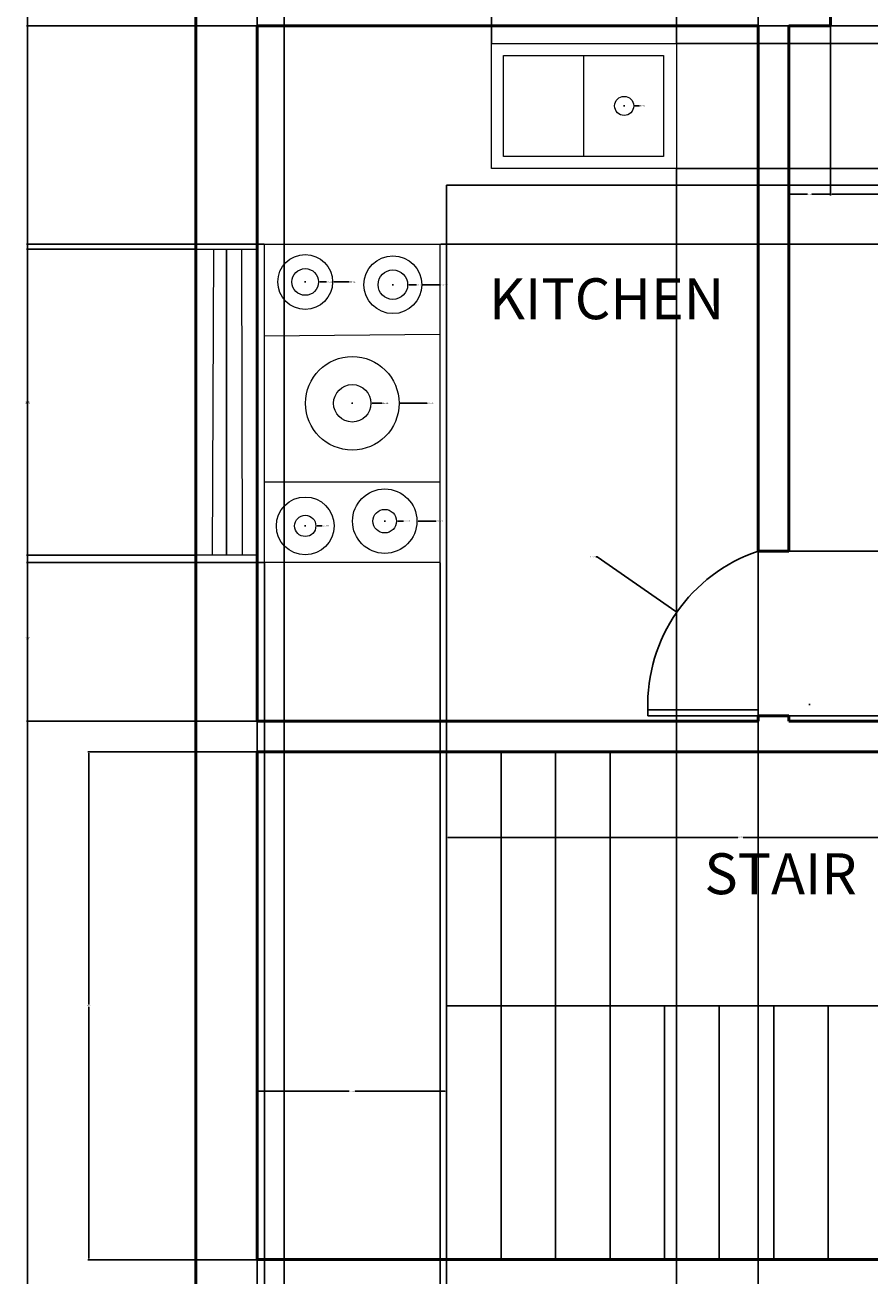
# Model space of a CAD drawing. Units: inches. Extents: x 1926 to 2293, y 1738 to 2280.
# Tile 3 of 6: x 1926 to 2050, y 1931 to 2114. Entities that reach past the tile are written whole.
import ezdxf

# ---------------------------------------------------------------- set-up
doc = ezdxf.new("R2010")
doc.units = ezdxf.units.IN
for name, color, linetype, lineweight in [('A-ANNO-DIMS', 2, 'Continuous', 18), ('A-AREA-IDEN', 7, 'Continuous', 25), ('A-DOOR', 3, 'Continuous', 25), ('A-EQPM', 8, 'Continuous', 18), ('A-FLOR-CASE', 9, 'Continuous', 25), ('A-FLOR-FIXT', 9, 'Continuous', 18), ('A-FLOR-STRS', 7, 'Continuous', 25), ('A-GLAZ', 4, 'Continuous', 18), ('A-WALL', 7, 'Continuous', 50)]:
    doc.layers.add(name, color=color, linetype=linetype, lineweight=lineweight)
doc.styles.get("Standard").update_dxf_attribs({"font": 'arial.ttf'})
doc.dimstyles.get("Standard").update_dxf_attribs({"dimtxt": 0.18, "dimasz": 0.18, "dimexe": 0.18, "dimexo": 0.0625, "dimgap": 0.09, "dimtad": 0, "dimtih": 1, "dimtoh": 1, "dimdec": 4, "dimzin": 0, "dimdsep": 46, "dimtxsty": 'Standard', "dimcen": 0.09, "dimadec": 0, "dimazin": 0, "dimtfac": 1, "dimtdec": 4, "dimtofl": 0, "dimtmove": 0, "dimatfit": 3, "dimfxl": 1, "dimtolj": 1, "dimtzin": 0, "dimarcsym": 0})

# ---------------------------------------------------------------- blocks, each defined once
blk = doc.blocks.new('*D39')
at = {"layer": 'A-ANNO-DIMS', "color": 0, "lineweight": -2, "transparency": 16777216}
for p, q in [((1959.69, 2007.66), (1934.88, 2007.66)), ((1935.06, 2007.48), (1935.06, 1970.59)), ((1935.06, 1933.34), (1935.06, 1970.23)), ((1959.69, 1933.16), (1934.88, 1933.16))]:
    blk.add_line(p, q, dxfattribs=at)
at = {"layer": 'A-ANNO-DIMS', "color": 0, "transparency": 16777216}
for points in [[(1935.03, 2007.48), (1935.09, 2007.48), (1935.06, 2007.66)], [(1935.03, 1933.34), (1935.09, 1933.34), (1935.06, 1933.16)]]:
    blk.add_solid(points, dxfattribs=at)
at = {"layer": 'Defpoints', "color": 0, "transparency": 16777216}
for p in [(1935.06, 2007.66), (1959.76, 2007.66), (1959.76, 1933.16)]:
    blk.add_point(p, dxfattribs=at)
at = {"layer": 'A-ANNO-DIMS', "color": 0, "transparency": 16777216, "insert": (1935.06, 1970.41), "char_height": 0.18, "attachment_point": 5}
blk.add_mtext('\\A1;74.5', dxfattribs=at)
blk = doc.blocks.new('*D40')
at = {"layer": 'A-ANNO-DIMS', "color": 0, "lineweight": -2, "transparency": 16777216}
for p, q in [((1959.69, 2114.16), (1925.88, 2114.16)), ((1926.06, 2113.98), (1926.06, 2063.34)), ((1926.06, 2012.34), (1926.06, 2062.98)), ((1959.69, 2012.16), (1925.88, 2012.16))]:
    blk.add_line(p, q, dxfattribs=at)
at = {"layer": 'A-ANNO-DIMS', "color": 0, "transparency": 16777216}
for points in [[(1926.03, 2113.98), (1926.09, 2113.98), (1926.06, 2114.16)], [(1926.03, 2012.34), (1926.09, 2012.34), (1926.06, 2012.16)]]:
    blk.add_solid(points, dxfattribs=at)
at = {"layer": 'Defpoints', "color": 0, "transparency": 16777216}
for p in [(1926.06, 2114.16), (1959.76, 2114.16), (1959.76, 2012.16)]:
    blk.add_point(p, dxfattribs=at)
at = {"layer": 'A-ANNO-DIMS', "color": 0, "transparency": 16777216, "insert": (1926.06, 2063.16), "char_height": 0.18, "attachment_point": 5}
blk.add_mtext('\\A1;102', dxfattribs=at)
blk = doc.blocks.new('*D46')
at = {"layer": 'A-ANNO-DIMS', "color": 0, "lineweight": -2, "transparency": 16777216}
for p, q in [((1959.76, 2114.22), (1959.76, 2280.04)), ((1959.94, 2279.86), (1996.18, 2279.86)), ((2033.08, 2279.86), (1996.83, 2279.86)), ((2033.26, 2114.22), (2033.26, 2280.04))]:
    blk.add_line(p, q, dxfattribs=at)
at = {"layer": 'A-ANNO-DIMS', "color": 0, "transparency": 16777216}
for points in [[(1959.94, 2279.89), (1959.94, 2279.83), (1959.76, 2279.86)], [(2033.08, 2279.89), (2033.08, 2279.83), (2033.26, 2279.86)]]:
    blk.add_solid(points, dxfattribs=at)
at = {"layer": 'Defpoints', "color": 0, "transparency": 16777216}
for p in [(2033.26, 2279.86), (1959.76, 2114.16), (2033.26, 2114.16)]:
    blk.add_point(p, dxfattribs=at)
at = {"layer": 'A-ANNO-DIMS', "color": 0, "transparency": 16777216, "insert": (1996.51, 2279.86), "char_height": 0.18, "attachment_point": 5}
blk.add_mtext('\\A1;73.5', dxfattribs=at)
blk = doc.blocks.new('*D47')
at = {"layer": 'A-ANNO-DIMS', "color": 0, "lineweight": -2, "transparency": 16777216}
for p, q in [((1950.76, 2036.47), (1950.76, 1737.97)), ((1959.76, 2036.47), (1959.76, 1737.97)), ((1950.94, 1738.15), (1955.11, 1738.15)), ((1959.58, 1738.15), (1955.41, 1738.15))]:
    blk.add_line(p, q, dxfattribs=at)
at = {"layer": 'A-ANNO-DIMS', "color": 0, "transparency": 16777216}
for points in [[(1950.94, 1738.18), (1950.94, 1738.12), (1950.76, 1738.15)], [(1959.58, 1738.18), (1959.58, 1738.12), (1959.76, 1738.15)]]:
    blk.add_solid(points, dxfattribs=at)
at = {"layer": 'Defpoints', "color": 0, "transparency": 16777216}
for p in [(1950.76, 2036.53), (1959.76, 2036.53), (1959.76, 1738.15)]:
    blk.add_point(p, dxfattribs=at)
at = {"layer": 'A-ANNO-DIMS', "color": 0, "transparency": 16777216, "insert": (1955.26, 1738.15), "char_height": 0.18, "attachment_point": 5}
blk.add_mtext('\\A1;9', dxfattribs=at)
blk = doc.blocks.new('*D48')
at = {"layer": 'A-ANNO-DIMS', "color": 0, "lineweight": -2, "transparency": 16777216}
for p, q in [((1950.69, 2036.53), (1925.88, 2036.53)), ((1926.06, 2036.35), (1926.06, 2024.53)), ((1926.06, 2012.34), (1926.06, 2024.16)), ((1959.69, 2012.16), (1925.88, 2012.16))]:
    blk.add_line(p, q, dxfattribs=at)
at = {"layer": 'A-ANNO-DIMS', "color": 0, "transparency": 16777216}
for points in [[(1926.03, 2036.35), (1926.09, 2036.35), (1926.06, 2036.53)], [(1926.03, 2012.34), (1926.09, 2012.34), (1926.06, 2012.16)]]:
    blk.add_solid(points, dxfattribs=at)
at = {"layer": 'Defpoints', "color": 0, "transparency": 16777216}
for p in [(1926.06, 2036.53), (1950.76, 2036.53), (1959.76, 2012.16)]:
    blk.add_point(p, dxfattribs=at)
at = {"layer": 'A-ANNO-DIMS', "color": 0, "transparency": 16777216, "insert": (1926.06, 2024.35), "char_height": 0.18, "attachment_point": 5}
blk.add_mtext('\\A1;24.367', dxfattribs=at)
blk = doc.blocks.new('*D49')
at = {"layer": 'A-ANNO-DIMS', "color": 0, "lineweight": -2, "transparency": 16777216}
for p, q in [((1950.69, 2081.42), (1925.88, 2081.42)), ((1926.06, 2081.24), (1926.06, 2059.16)), ((1926.06, 2036.71), (1926.06, 2058.79)), ((1950.69, 2036.53), (1925.88, 2036.53))]:
    blk.add_line(p, q, dxfattribs=at)
at = {"layer": 'A-ANNO-DIMS', "color": 0, "transparency": 16777216}
for points in [[(1926.03, 2081.24), (1926.09, 2081.24), (1926.06, 2081.42)], [(1926.03, 2036.71), (1926.09, 2036.71), (1926.06, 2036.53)]]:
    blk.add_solid(points, dxfattribs=at)
at = {"layer": 'Defpoints', "color": 0, "transparency": 16777216}
for p in [(1926.06, 2081.42), (1950.76, 2081.42), (1950.76, 2036.53)]:
    blk.add_point(p, dxfattribs=at)
at = {"layer": 'A-ANNO-DIMS', "color": 0, "transparency": 16777216, "insert": (1926.06, 2058.98), "char_height": 0.18, "attachment_point": 5}
blk.add_mtext('\\A1;44.89', dxfattribs=at)
blk = doc.blocks.new('*D50')
at = {"layer": 'A-ANNO-DIMS', "color": 0, "lineweight": -2, "transparency": 16777216}
for p, q in [((2033.32, 2037.09), (2281.64, 2037.09)), ((2281.46, 2036.91), (2281.46, 2025.19)), ((2281.46, 2013.1), (2281.46, 2024.83)), ((2033.32, 2012.92), (2281.64, 2012.92))]:
    blk.add_line(p, q, dxfattribs=at)
at = {"layer": 'A-ANNO-DIMS', "color": 0, "transparency": 16777216}
for points in [[(2281.43, 2036.91), (2281.49, 2036.91), (2281.46, 2037.09)], [(2281.43, 2013.1), (2281.49, 2013.1), (2281.46, 2012.92)]]:
    blk.add_solid(points, dxfattribs=at)
at = {"layer": 'Defpoints', "color": 0, "transparency": 16777216}
for p in [(2033.26, 2037.09), (2281.46, 2037.09), (2033.26, 2012.92)]:
    blk.add_point(p, dxfattribs=at)
at = {"layer": 'A-ANNO-DIMS', "color": 0, "transparency": 16777216, "insert": (2281.46, 2025.01), "char_height": 0.18, "attachment_point": 5}
blk.add_mtext('\\A1;24.17', dxfattribs=at)
blk = doc.blocks.new('*D51')
at = {"layer": 'A-ANNO-DIMS', "color": 0, "lineweight": -2, "transparency": 16777216}
for p, q in [((1959.76, 2012.1), (1959.76, 1737.97)), ((1987.52, 2012.1), (1987.52, 1737.97)), ((1959.94, 1738.15), (1973.24, 1738.15)), ((1987.34, 1738.15), (1974.03, 1738.15))]:
    blk.add_line(p, q, dxfattribs=at)
at = {"layer": 'A-ANNO-DIMS', "color": 0, "transparency": 16777216}
for points in [[(1959.94, 1738.18), (1959.94, 1738.12), (1959.76, 1738.15)], [(1987.34, 1738.18), (1987.34, 1738.12), (1987.52, 1738.15)]]:
    blk.add_solid(points, dxfattribs=at)
at = {"layer": 'Defpoints', "color": 0, "transparency": 16777216}
for p in [(1959.76, 2012.16), (1987.52, 2012.16), (1987.52, 1738.15)]:
    blk.add_point(p, dxfattribs=at)
at = {"layer": 'A-ANNO-DIMS', "color": 0, "transparency": 16777216, "insert": (1973.64, 1738.15), "char_height": 0.18, "attachment_point": 5}
blk.add_mtext('\\A1;27.76', dxfattribs=at)
blk = doc.blocks.new('*D52')
at = {"layer": 'A-ANNO-DIMS', "color": 0, "lineweight": -2, "transparency": 16777216}
for p, q in [((2033.32, 2114.16), (2281.64, 2114.16)), ((2281.46, 2113.98), (2281.46, 2102.67)), ((2281.46, 2090.99), (2281.46, 2102.31)), ((2033.32, 2090.81), (2281.64, 2090.81))]:
    blk.add_line(p, q, dxfattribs=at)
at = {"layer": 'A-ANNO-DIMS', "color": 0, "transparency": 16777216}
for points in [[(2281.43, 2113.98), (2281.49, 2113.98), (2281.46, 2114.16)], [(2281.43, 2090.99), (2281.49, 2090.99), (2281.46, 2090.81)]]:
    blk.add_solid(points, dxfattribs=at)
at = {"layer": 'Defpoints', "color": 0, "transparency": 16777216}
for p in [(2033.26, 2114.16), (2281.46, 2114.16), (2033.26, 2090.81)]:
    blk.add_point(p, dxfattribs=at)
at = {"layer": 'A-ANNO-DIMS', "color": 0, "transparency": 16777216, "insert": (2281.46, 2102.49), "char_height": 0.18, "attachment_point": 5}
blk.add_mtext('\\A1;23.348', dxfattribs=at)
blk = doc.blocks.new('*D53')
at = {"layer": 'A-ANNO-DIMS', "color": 0, "lineweight": -2, "transparency": 16777216}
for p, q in [((1994.13, 2111.62), (1994.13, 2280.04)), ((1994.31, 2279.86), (2007.3, 2279.86)), ((2021.07, 2279.86), (2008.09, 2279.86)), ((2021.25, 2111.62), (2021.25, 2280.04))]:
    blk.add_line(p, q, dxfattribs=at)
at = {"layer": 'A-ANNO-DIMS', "color": 0, "transparency": 16777216}
for points in [[(1994.31, 2279.89), (1994.31, 2279.83), (1994.13, 2279.86)], [(2021.07, 2279.89), (2021.07, 2279.83), (2021.25, 2279.86)]]:
    blk.add_solid(points, dxfattribs=at)
at = {"layer": 'Defpoints', "color": 0, "transparency": 16777216}
for p in [(2021.25, 2279.86), (1994.13, 2111.56), (2021.25, 2111.56)]:
    blk.add_point(p, dxfattribs=at)
at = {"layer": 'A-ANNO-DIMS', "color": 0, "transparency": 16777216, "insert": (2007.69, 2279.86), "char_height": 0.18, "attachment_point": 5}
blk.add_mtext('\\A1;27.13', dxfattribs=at)
blk = doc.blocks.new('*D54')
at = {"layer": 'A-ANNO-DIMS', "color": 0, "lineweight": -2, "transparency": 16777216}
for p, q in [((2021.32, 2111.56), (2281.64, 2111.56)), ((2281.46, 2111.38), (2281.46, 2102.58)), ((2281.46, 2093.41), (2281.46, 2102.21)), ((2021.32, 2093.23), (2281.64, 2093.23))]:
    blk.add_line(p, q, dxfattribs=at)
at = {"layer": 'A-ANNO-DIMS', "color": 0, "transparency": 16777216}
for points in [[(2281.43, 2111.38), (2281.49, 2111.38), (2281.46, 2111.56)], [(2281.43, 2093.41), (2281.49, 2093.41), (2281.46, 2093.23)]]:
    blk.add_solid(points, dxfattribs=at)
at = {"layer": 'Defpoints', "color": 0, "transparency": 16777216}
for p in [(2021.25, 2111.56), (2281.46, 2111.56), (2021.25, 2093.23)]:
    blk.add_point(p, dxfattribs=at)
at = {"layer": 'A-ANNO-DIMS', "color": 0, "transparency": 16777216, "insert": (2281.46, 2102.39), "char_height": 0.18, "attachment_point": 5}
blk.add_mtext('\\A1;18.332', dxfattribs=at)
blk = doc.blocks.new('*D55')
at = {"layer": 'A-ANNO-DIMS', "color": 0, "lineweight": -2, "transparency": 16777216}
for p, q in [((1960.83, 2035.38), (1960.83, 1737.97)), ((1986.57, 2035.38), (1986.57, 1737.97)), ((1961.01, 1738.15), (1973.3, 1738.15)), ((1986.39, 1738.15), (1974.09, 1738.15))]:
    blk.add_line(p, q, dxfattribs=at)
at = {"layer": 'A-ANNO-DIMS', "color": 0, "transparency": 16777216}
for points in [[(1961.01, 1738.18), (1961.01, 1738.12), (1960.83, 1738.15)], [(1986.39, 1738.18), (1986.39, 1738.12), (1986.57, 1738.15)]]:
    blk.add_solid(points, dxfattribs=at)
at = {"layer": 'Defpoints', "color": 0, "transparency": 16777216}
for p in [(1960.83, 2035.45), (1986.57, 2035.45), (1986.57, 1738.15)]:
    blk.add_point(p, dxfattribs=at)
at = {"layer": 'A-ANNO-DIMS', "color": 0, "transparency": 16777216, "insert": (1973.7, 1738.15), "char_height": 0.18, "attachment_point": 5}
blk.add_mtext('\\A1;25.74', dxfattribs=at)
blk = doc.blocks.new('*D56')
at = {"layer": 'A-ANNO-DIMS', "color": 0, "lineweight": -2, "transparency": 16777216}
for p, q in [((1960.76, 2082.13), (1925.88, 2082.13)), ((1926.06, 2081.95), (1926.06, 2058.97)), ((1926.06, 2035.63), (1926.06, 2058.61)), ((1960.76, 2035.45), (1925.88, 2035.45))]:
    blk.add_line(p, q, dxfattribs=at)
at = {"layer": 'A-ANNO-DIMS', "color": 0, "transparency": 16777216}
for points in [[(1926.03, 2081.95), (1926.09, 2081.95), (1926.06, 2082.13)], [(1926.03, 2035.63), (1926.09, 2035.63), (1926.06, 2035.45)]]:
    blk.add_solid(points, dxfattribs=at)
at = {"layer": 'Defpoints', "color": 0, "transparency": 16777216}
for p in [(1926.06, 2082.13), (1960.83, 2082.13), (1960.83, 2035.45)]:
    blk.add_point(p, dxfattribs=at)
at = {"layer": 'A-ANNO-DIMS', "color": 0, "transparency": 16777216, "insert": (1926.06, 2058.79), "char_height": 0.18, "attachment_point": 5}
blk.add_mtext('\\A1;46.69', dxfattribs=at)
blk = doc.blocks.new('*D57')
at = {"layer": 'A-ANNO-DIMS', "color": 0, "lineweight": -2, "transparency": 16777216}
for p, q in [((2021.25, 2093.16), (2021.25, 1737.97)), ((2033.26, 2090.75), (2033.26, 1737.97)), ((2021.43, 1738.15), (2026.8, 1738.15)), ((2033.08, 1738.15), (2027.71, 1738.15))]:
    blk.add_line(p, q, dxfattribs=at)
at = {"layer": 'A-ANNO-DIMS', "color": 0, "transparency": 16777216}
for points in [[(2021.43, 1738.18), (2021.43, 1738.12), (2021.25, 1738.15)], [(2033.08, 1738.18), (2033.08, 1738.12), (2033.26, 1738.15)]]:
    blk.add_solid(points, dxfattribs=at)
at = {"layer": 'Defpoints', "color": 0, "transparency": 16777216}
for p in [(2021.25, 2093.23), (2033.26, 2090.81), (2033.26, 1738.15)]:
    blk.add_point(p, dxfattribs=at)
at = {"layer": 'A-ANNO-DIMS', "color": 0, "transparency": 16777216, "insert": (2027.26, 1738.15), "char_height": 0.18, "attachment_point": 5}
blk.add_mtext('\\A1;12.002', dxfattribs=at)
blk = doc.blocks.new('*D58')
at = {"layer": 'A-ANNO-DIMS', "color": 0, "lineweight": -2, "transparency": 16777216}
for p, q in [((1987.58, 2090.81), (2281.64, 2090.81)), ((2281.46, 2090.63), (2281.46, 2086.66)), ((2281.46, 2082.31), (2281.46, 2086.29)), ((1986.63, 2082.13), (2281.64, 2082.13))]:
    blk.add_line(p, q, dxfattribs=at)
at = {"layer": 'A-ANNO-DIMS', "color": 0, "transparency": 16777216}
for points in [[(2281.43, 2090.63), (2281.49, 2090.63), (2281.46, 2090.81)], [(2281.43, 2082.31), (2281.49, 2082.31), (2281.46, 2082.13)]]:
    blk.add_solid(points, dxfattribs=at)
at = {"layer": 'Defpoints', "color": 0, "transparency": 16777216}
for p in [(1987.52, 2090.81), (2281.46, 2090.81), (1986.57, 2082.13)]:
    blk.add_point(p, dxfattribs=at)
at = {"layer": 'A-ANNO-DIMS', "color": 0, "transparency": 16777216, "insert": (2281.46, 2086.47), "char_height": 0.18, "attachment_point": 5}
blk.add_mtext('\\A1;8.682', dxfattribs=at)
blk = doc.blocks.new('*D63')
at = {"layer": 'A-ANNO-DIMS', "color": 0, "lineweight": -2, "transparency": 16777216}
for p, q in [((2043.88, 2114.1), (2043.88, 2089.28)), ((2073.61, 2114.1), (2073.61, 2089.28)), ((2044.06, 2089.46), (2058.35, 2089.46)), ((2073.43, 2089.46), (2059.14, 2089.46))]:
    blk.add_line(p, q, dxfattribs=at)
at = {"layer": 'A-ANNO-DIMS', "color": 0, "transparency": 16777216}
for points in [[(2044.06, 2089.49), (2044.06, 2089.43), (2043.88, 2089.46)], [(2073.43, 2089.49), (2073.43, 2089.43), (2073.61, 2089.46)]]:
    blk.add_solid(points, dxfattribs=at)
at = {"layer": 'Defpoints', "color": 0, "transparency": 16777216}
for p in [(2043.88, 2114.16), (2073.61, 2114.16), (2043.88, 2089.46)]:
    blk.add_point(p, dxfattribs=at)
at = {"layer": 'A-ANNO-DIMS', "color": 0, "transparency": 16777216, "insert": (2058.74, 2089.46), "char_height": 0.18, "attachment_point": 5}
blk.add_mtext('\\A1;29.73', dxfattribs=at)
blk = doc.blocks.new('*D64')
at = {"layer": 'A-ANNO-DIMS', "color": 0, "lineweight": -2, "transparency": 16777216}
for p, q in [((2037.76, 2114.1), (2037.76, 2089.28)), ((2043.88, 2114.1), (2043.88, 2089.28)), ((2037.94, 2089.46), (2040.49, 2089.46)), ((2043.7, 2089.46), (2041.14, 2089.46))]:
    blk.add_line(p, q, dxfattribs=at)
at = {"layer": 'A-ANNO-DIMS', "color": 0, "transparency": 16777216}
for points in [[(2037.94, 2089.49), (2037.94, 2089.43), (2037.76, 2089.46)], [(2043.7, 2089.49), (2043.7, 2089.43), (2043.88, 2089.46)]]:
    blk.add_solid(points, dxfattribs=at)
at = {"layer": 'Defpoints', "color": 0, "transparency": 16777216}
for p in [(2037.76, 2114.16), (2043.88, 2114.16), (2037.76, 2089.46)]:
    blk.add_point(p, dxfattribs=at)
at = {"layer": 'A-ANNO-DIMS', "color": 0, "transparency": 16777216, "insert": (2040.82, 2089.46), "char_height": 0.18, "attachment_point": 5}
blk.add_mtext('\\A1;6.12', dxfattribs=at)
blk = doc.blocks.new('*D68')
at = {"layer": 'A-ANNO-DIMS', "color": 0, "lineweight": -2, "transparency": 16777216}
for p, q in [((1959.76, 1933.22), (1959.76, 1958.04)), ((1959.94, 1957.86), (1973.18, 1957.86)), ((1987.35, 1957.86), (1974.11, 1957.86)), ((1987.53, 1933.22), (1987.53, 1958.04))]:
    blk.add_line(p, q, dxfattribs=at)
at = {"layer": 'A-ANNO-DIMS', "color": 0, "transparency": 16777216}
for points in [[(1959.94, 1957.89), (1959.94, 1957.83), (1959.76, 1957.86)], [(1987.35, 1957.89), (1987.35, 1957.83), (1987.53, 1957.86)]]:
    blk.add_solid(points, dxfattribs=at)
at = {"layer": 'Defpoints', "color": 0, "transparency": 16777216}
for p in [(1987.53, 1957.86), (1959.76, 1933.16), (1987.53, 1933.16)]:
    blk.add_point(p, dxfattribs=at)
at = {"layer": 'A-ANNO-DIMS', "color": 0, "transparency": 16777216, "insert": (1973.64, 1957.86), "char_height": 0.18, "attachment_point": 5}
blk.add_mtext('\\A1;27.774', dxfattribs=at)
blk = doc.blocks.new('*D69')
at = {"layer": 'A-ANNO-DIMS', "color": 0, "lineweight": -2, "transparency": 16777216}
for p, q in [((1987.53, 1970.47), (1987.53, 1995.29)), ((2073.75, 1970.47), (2073.75, 1995.29)), ((1987.71, 1995.11), (2030.25, 1995.11)), ((2073.57, 1995.11), (2031.03, 1995.11))]:
    blk.add_line(p, q, dxfattribs=at)
at = {"layer": 'A-ANNO-DIMS', "color": 0, "transparency": 16777216}
for points in [[(1987.71, 1995.14), (1987.71, 1995.08), (1987.53, 1995.11)], [(2073.57, 1995.14), (2073.57, 1995.08), (2073.75, 1995.11)]]:
    blk.add_solid(points, dxfattribs=at)
at = {"layer": 'Defpoints', "color": 0, "transparency": 16777216}
for p in [(2073.75, 1995.11), (1987.53, 1970.41), (2073.75, 1970.41)]:
    blk.add_point(p, dxfattribs=at)
at = {"layer": 'A-ANNO-DIMS', "color": 0, "transparency": 16777216, "insert": (2030.64, 1995.11), "char_height": 0.18, "attachment_point": 5}
blk.add_mtext('\\A1;86.22', dxfattribs=at)
blk = doc.blocks.new('*D79')
at = {"layer": 'A-ANNO-DIMS', "color": 0, "lineweight": -2, "transparency": 16777216}
for p, q in [((1959.76, 1833.35), (1959.76, 2280.04)), ((1959.94, 2279.86), (1961.41, 2279.86)), ((1963.53, 2279.86), (1962.06, 2279.86)), ((1963.71, 1828.81), (1963.71, 2280.04))]:
    blk.add_line(p, q, dxfattribs=at)
at = {"layer": 'A-ANNO-DIMS', "color": 0, "transparency": 16777216}
for points in [[(1959.94, 2279.89), (1959.94, 2279.83), (1959.76, 2279.86)], [(1963.53, 2279.89), (1963.53, 2279.83), (1963.71, 2279.86)]]:
    blk.add_solid(points, dxfattribs=at)
at = {"layer": 'Defpoints', "color": 0, "transparency": 16777216}
for p in [(1959.76, 2279.86), (1959.76, 1833.29), (1963.71, 1828.75)]:
    blk.add_point(p, dxfattribs=at)
at = {"layer": 'A-ANNO-DIMS', "color": 0, "transparency": 16777216, "insert": (1961.74, 2279.86), "char_height": 0.18, "attachment_point": 5}
blk.add_mtext('\\A1;3.96', dxfattribs=at)
blk = doc.blocks.new('*D85')
at = {"layer": 'A-ANNO-DIMS', "color": 0, "lineweight": -2, "transparency": 16777216}
for p, q in [((1950.69, 2255.16), (1925.88, 2255.16)), ((1926.06, 2254.98), (1926.06, 2024.34)), ((1926.06, 1793.34), (1926.06, 2023.98)), ((1950.69, 1793.16), (1925.88, 1793.16))]:
    blk.add_line(p, q, dxfattribs=at)
at = {"layer": 'A-ANNO-DIMS', "color": 0, "transparency": 16777216}
for points in [[(1926.03, 2254.98), (1926.09, 2254.98), (1926.06, 2255.16)], [(1926.03, 1793.34), (1926.09, 1793.34), (1926.06, 1793.16)]]:
    blk.add_solid(points, dxfattribs=at)
at = {"layer": 'Defpoints', "color": 0, "transparency": 16777216}
for p in [(1926.06, 2255.16), (1950.76, 2255.16), (1950.76, 1793.16)]:
    blk.add_point(p, dxfattribs=at)
at = {"layer": 'A-ANNO-DIMS', "color": 0, "transparency": 16777216, "insert": (1926.06, 2024.16), "char_height": 0.18, "attachment_point": 5}
blk.add_mtext('\\A1;462', dxfattribs=at)
blk = doc.blocks.new('*D88')
at = {"layer": 'A-ANNO-DIMS', "color": 0, "lineweight": -2, "transparency": 16777216}
for p, q in [((2072.97, 1939.43), (2073.15, 1939.43)), ((2073.06, 1939.34), (2073.06, 1939.52)), ((2043.15, 1883.11), (2054.28, 1904.07)), ((2042.97, 1883.11), (2043.15, 1883.11))]:
    blk.add_line(p, q, dxfattribs=at)
at = {"layer": 'A-ANNO-DIMS', "color": 0, "transparency": 16777216}
blk.add_solid([(2054.26, 1904.08), (2054.31, 1904.06), (2054.37, 1904.23)], dxfattribs=at)
at = {"layer": 'Defpoints', "color": 0, "transparency": 16777216}
for p in [(2073.06, 1939.43), (2054.37, 1904.23)]:
    blk.add_point(p, dxfattribs=at)
at = {"layer": 'A-ANNO-DIMS', "color": 0, "transparency": 16777216, "insert": (2042.49, 1883.11), "char_height": 0.18, "attachment_point": 5}
blk.add_mtext('\\A1;R39.85', dxfattribs=at)
blk = doc.blocks.new('*D91')
at = {"layer": 'A-ANNO-DIMS', "color": 0, "lineweight": -2, "transparency": 16777216}
for p, q in [((2009.43, 2036.26), (2009.61, 2036.26)), ((2009.61, 2036.26), (2021.15, 2028.24)), ((2040.69, 2014.59), (2040.87, 2014.59)), ((2040.78, 2014.5), (2040.78, 2014.68))]:
    blk.add_line(p, q, dxfattribs=at)
at = {"layer": 'A-ANNO-DIMS', "color": 0, "transparency": 16777216}
blk.add_solid([(2021.17, 2028.26), (2021.13, 2028.21), (2021.3, 2028.13)], dxfattribs=at)
at = {"layer": 'Defpoints', "color": 0, "transparency": 16777216}
for p in [(2021.3, 2028.13), (2040.78, 2014.59)]:
    blk.add_point(p, dxfattribs=at)
at = {"layer": 'A-ANNO-DIMS', "color": 0, "transparency": 16777216, "insert": (2008.95, 2036.26), "char_height": 0.18, "attachment_point": 5}
blk.add_mtext('\\A1;R23.72', dxfattribs=at)
blk = doc.blocks.new('*D93')
at = {"layer": 'A-ANNO-DIMS', "color": 0, "lineweight": -2, "transparency": 16777216}
for p, q in [((1973.61, 2058.79), (1973.79, 2058.79)), ((1973.7, 2058.7), (1973.7, 2058.88)), ((1984.67, 2058.79), (1980.74, 2058.79))]:
    blk.add_line(p, q, dxfattribs=at)
at = {"layer": 'A-ANNO-DIMS', "color": 0, "transparency": 16777216}
blk.add_solid([(1980.74, 2058.82), (1980.74, 2058.76), (1980.56, 2058.79)], dxfattribs=at)
at = {"layer": 'Defpoints', "color": 0, "transparency": 16777216}
for p in [(1966.84, 2058.79), (1980.56, 2058.79)]:
    blk.add_point(p, dxfattribs=at)
at = {"layer": 'A-ANNO-DIMS', "color": 0, "transparency": 16777216, "insert": (1985.16, 2058.79), "char_height": 0.18, "attachment_point": 5}
blk.add_mtext('\\A1;∅13.72', dxfattribs=at)
blk = doc.blocks.new('*D94')
at = {"layer": 'A-ANNO-DIMS', "color": 0, "lineweight": -2, "transparency": 16777216}
for p, q in [((2013.5, 2102.42), (2013.68, 2102.42)), ((2013.59, 2102.33), (2013.59, 2102.51)), ((2015.83, 2102.45), (2015.17, 2102.44))]:
    blk.add_line(p, q, dxfattribs=at)
at = {"layer": 'A-ANNO-DIMS', "color": 0, "transparency": 16777216}
blk.add_solid([(2015.17, 2102.47), (2015.17, 2102.41), (2014.99, 2102.44)], dxfattribs=at)
at = {"layer": 'Defpoints', "color": 0, "transparency": 16777216}
for p in [(2012.19, 2102.4), (2014.99, 2102.44)]:
    blk.add_point(p, dxfattribs=at)
at = {"layer": 'A-ANNO-DIMS', "color": 0, "transparency": 16777216, "insert": (2016.26, 2102.45), "char_height": 0.18, "attachment_point": 5}
blk.add_mtext('\\A1;∅2.80', dxfattribs=at)
blk = doc.blocks.new('*D95')
at = {"layer": 'A-ANNO-DIMS', "color": 0, "lineweight": -2, "transparency": 16777216}
for p, q in [((1966.7, 2076.59), (1966.88, 2076.59)), ((1966.79, 2076.5), (1966.79, 2076.68)), ((1973.23, 2076.59), (1971, 2076.59))]:
    blk.add_line(p, q, dxfattribs=at)
at = {"layer": 'A-ANNO-DIMS', "color": 0, "transparency": 16777216}
blk.add_solid([(1971, 2076.62), (1971, 2076.56), (1970.82, 2076.59)], dxfattribs=at)
at = {"layer": 'Defpoints', "color": 0, "transparency": 16777216}
for p in [(1962.77, 2076.59), (1970.82, 2076.59)]:
    blk.add_point(p, dxfattribs=at)
at = {"layer": 'A-ANNO-DIMS', "color": 0, "transparency": 16777216, "insert": (1973.72, 2076.59), "char_height": 0.18, "attachment_point": 5}
blk.add_mtext('\\A1;∅8.044', dxfattribs=at)
blk = doc.blocks.new('*D96')
at = {"layer": 'A-ANNO-DIMS', "color": 0, "lineweight": -2, "transparency": 16777216}
for p, q in [((1966.7, 2076.59), (1966.88, 2076.59)), ((1966.79, 2076.5), (1966.79, 2076.68)), ((1969.93, 2076.59), (1968.93, 2076.59))]:
    blk.add_line(p, q, dxfattribs=at)
at = {"layer": 'A-ANNO-DIMS', "color": 0, "transparency": 16777216}
blk.add_solid([(1968.93, 2076.62), (1968.93, 2076.56), (1968.75, 2076.59)], dxfattribs=at)
at = {"layer": 'Defpoints', "color": 0, "transparency": 16777216}
for p in [(1964.84, 2076.59), (1968.75, 2076.59)]:
    blk.add_point(p, dxfattribs=at)
at = {"layer": 'A-ANNO-DIMS', "color": 0, "transparency": 16777216, "insert": (1970.42, 2076.59), "char_height": 0.18, "attachment_point": 5}
blk.add_mtext('\\A1;∅3.916', dxfattribs=at)
blk = doc.blocks.new('*D97')
at = {"layer": 'A-ANNO-DIMS', "color": 0, "lineweight": -2, "transparency": 16777216}
for p, q in [((1979.57, 2076.19), (1979.75, 2076.19)), ((1979.66, 2076.1), (1979.66, 2076.28)), ((1986.44, 2076.17), (1984.07, 2076.18))]:
    blk.add_line(p, q, dxfattribs=at)
at = {"layer": 'A-ANNO-DIMS', "color": 0, "transparency": 16777216}
blk.add_solid([(1984.07, 2076.21), (1984.07, 2076.15), (1983.89, 2076.18)], dxfattribs=at)
at = {"layer": 'Defpoints', "color": 0, "transparency": 16777216}
for p in [(1975.42, 2076.2), (1983.89, 2076.18)]:
    blk.add_point(p, dxfattribs=at)
at = {"layer": 'A-ANNO-DIMS', "color": 0, "transparency": 16777216, "insert": (1987.12, 2076.17), "char_height": 0.18, "attachment_point": 5}
blk.add_mtext('\\A1;2X ∅8.478', dxfattribs=at)
blk = doc.blocks.new('*D98')
at = {"layer": 'A-ANNO-DIMS', "color": 0, "lineweight": -2, "transparency": 16777216}
for p, q in [((1979.57, 2076.19), (1979.75, 2076.19)), ((1979.66, 2076.1), (1979.66, 2076.28)), ((1983.12, 2076.17), (1982, 2076.18))]:
    blk.add_line(p, q, dxfattribs=at)
at = {"layer": 'A-ANNO-DIMS', "color": 0, "transparency": 16777216}
blk.add_solid([(1982, 2076.21), (1982, 2076.15), (1981.82, 2076.18)], dxfattribs=at)
at = {"layer": 'Defpoints', "color": 0, "transparency": 16777216}
for p in [(1977.49, 2076.2), (1981.82, 2076.18)]:
    blk.add_point(p, dxfattribs=at)
at = {"layer": 'A-ANNO-DIMS', "color": 0, "transparency": 16777216, "insert": (1983.62, 2076.17), "char_height": 0.18, "attachment_point": 5}
blk.add_mtext('\\A1;∅4.335', dxfattribs=at)
blk = doc.blocks.new('*D99')
at = {"layer": 'A-ANNO-DIMS', "color": 0, "lineweight": -2, "transparency": 16777216}
for p, q in [((1973.61, 2058.79), (1973.79, 2058.79)), ((1973.7, 2058.7), (1973.7, 2058.88)), ((1978.09, 2058.79), (1976.62, 2058.79))]:
    blk.add_line(p, q, dxfattribs=at)
at = {"layer": 'A-ANNO-DIMS', "color": 0, "transparency": 16777216}
blk.add_solid([(1976.62, 2058.82), (1976.62, 2058.76), (1976.44, 2058.79)], dxfattribs=at)
at = {"layer": 'Defpoints', "color": 0, "transparency": 16777216}
for p in [(1970.95, 2058.79), (1976.44, 2058.79)]:
    blk.add_point(p, dxfattribs=at)
at = {"layer": 'A-ANNO-DIMS', "color": 0, "transparency": 16777216, "insert": (1978.56, 2058.79), "char_height": 0.18, "attachment_point": 5}
blk.add_mtext('\\A1;∅5.491', dxfattribs=at)
blk = doc.blocks.new('*D100')
at = {"layer": 'A-ANNO-DIMS', "color": 0, "lineweight": -2, "transparency": 16777216}
for p, q in [((1966.71, 2040.8), (1966.89, 2040.8)), ((1966.8, 2040.71), (1966.8, 2040.89)), ((1969.29, 2040.83), (1968.53, 2040.82))]:
    blk.add_line(p, q, dxfattribs=at)
at = {"layer": 'A-ANNO-DIMS', "color": 0, "transparency": 16777216}
blk.add_solid([(1968.53, 2040.85), (1968.53, 2040.79), (1968.35, 2040.82)], dxfattribs=at)
at = {"layer": 'Defpoints', "color": 0, "transparency": 16777216}
for p in [(1965.24, 2040.78), (1968.35, 2040.82)]:
    blk.add_point(p, dxfattribs=at)
at = {"layer": 'A-ANNO-DIMS', "color": 0, "transparency": 16777216, "insert": (1969.78, 2040.83), "char_height": 0.18, "attachment_point": 5}
blk.add_mtext('\\A1;∅3.114', dxfattribs=at)
blk = doc.blocks.new('*D101')
at = {"layer": 'A-ANNO-DIMS', "color": 0, "lineweight": -2, "transparency": 16777216}
for p, q in [((1978.37, 2041.5), (1978.55, 2041.5)), ((1978.46, 2041.41), (1978.46, 2041.59)), ((1986.02, 2041.52), (1983.36, 2041.51))]:
    blk.add_line(p, q, dxfattribs=at)
at = {"layer": 'A-ANNO-DIMS', "color": 0, "transparency": 16777216}
blk.add_solid([(1983.36, 2041.54), (1983.36, 2041.48), (1983.18, 2041.51)], dxfattribs=at)
at = {"layer": 'Defpoints', "color": 0, "transparency": 16777216}
for p in [(1973.74, 2041.49), (1983.18, 2041.51)]:
    blk.add_point(p, dxfattribs=at)
at = {"layer": 'A-ANNO-DIMS', "color": 0, "transparency": 16777216, "insert": (1986.51, 2041.52), "char_height": 0.18, "attachment_point": 5}
blk.add_mtext('\\A1;∅9.444', dxfattribs=at)
blk = doc.blocks.new('*D102')
at = {"layer": 'A-ANNO-DIMS', "color": 0, "lineweight": -2, "transparency": 16777216}
for p, q in [((1978.37, 2041.5), (1978.55, 2041.5)), ((1978.46, 2041.41), (1978.46, 2041.59)), ((1981.23, 2041.52), (1980.37, 2041.51))]:
    blk.add_line(p, q, dxfattribs=at)
at = {"layer": 'A-ANNO-DIMS', "color": 0, "transparency": 16777216}
blk.add_solid([(1980.37, 2041.54), (1980.37, 2041.48), (1980.19, 2041.51)], dxfattribs=at)
at = {"layer": 'Defpoints', "color": 0, "transparency": 16777216}
for p in [(1976.73, 2041.49), (1980.19, 2041.51)]:
    blk.add_point(p, dxfattribs=at)
at = {"layer": 'A-ANNO-DIMS', "color": 0, "transparency": 16777216, "insert": (1981.72, 2041.52), "char_height": 0.18, "attachment_point": 5}
blk.add_mtext('\\A1;∅3.459', dxfattribs=at)

msp = doc.modelspace()

# ---------------------------------------------------------------- linework, layer by layer
at = {"layer": 'A-DOOR'}
for p, q in [((2017.0689, 2012.9217), (2017.0689, 2013.8047)), ((2017.0689, 2013.8047), (2033.2569, 2013.8047)), ((2033.2569, 2013.8047), (2033.2569, 2012.9217)), ((2033.2569, 2012.9217), (2017.0689, 2012.9217))]:
    msp.add_line(p, q, dxfattribs=at)
msp.add_arc((2040.7776, 2014.5946), 23.7219, 108.483967, 181.908063, dxfattribs=at)
at = {"layer": 'A-EQPM'}
for p, q in [((1960.8266, 2068.7118), (1986.5655, 2068.911)), ((1960.8266, 2047.2934), (1986.5655, 2047.2934))]:
    msp.add_line(p, q, dxfattribs=at)
msp.add_lwpolyline([(1960.8266, 2082.133), (1986.5655, 2082.133), (1986.5655, 2035.4453), (1960.8266, 2035.4453)], close=True, dxfattribs=at)
for centre, radius in [((1966.7946, 2076.5885), 4.0222), ((1979.6559, 2076.19), 4.2388), ((1966.7946, 2076.5885), 1.9581), ((1979.6559, 2076.19), 2.1674), ((1973.696, 2058.7891), 6.8607), ((1973.696, 2058.7891), 2.7456), ((1966.7969, 2040.8011), 4.2388), ((1978.4618, 2041.4985), 4.722), ((1978.4618, 2041.4985), 1.7297), ((1966.7969, 2040.8011), 1.5571)]:
    msp.add_circle(centre, radius, dxfattribs=at)
at = {"layer": 'A-FLOR-CASE'}
for p, q in [((1987.5186, 2012.1622), (1987.5186, 2090.8146)), ((1987.5186, 2090.8146), (2033.2569, 2090.8146))]:
    msp.add_line(p, q, dxfattribs=at)
at = {"layer": 'A-FLOR-FIXT'}
msp.add_line((2007.624, 2109.8164), (2007.624, 2095.0195), dxfattribs=at)
for points in [[(1994.1266, 2111.5596), (2021.2546, 2111.5596), (2021.2546, 2093.2275), (1994.1266, 2093.2275)], [(1995.8924, 2109.8164), (2019.3556, 2109.8164), (2019.3556, 2095.0195), (1995.8924, 2095.0195)]]:
    msp.add_lwpolyline(points, close=True, dxfattribs=at)
msp.add_circle((2013.5904, 2102.418), 1.4023, dxfattribs=at)
at = {"layer": 'A-FLOR-STRS'}
for p, q in [((1987.531, 2007.6622), (1987.531, 1933.1622)), ((1995.531, 2007.6622), (1995.531, 1933.1622)), ((2003.531, 2007.6622), (2003.531, 1933.1622)), ((2011.531, 2007.6622), (2011.531, 1933.1622)), ((1987.531, 1970.4122), (2073.7521, 1970.4122)), ((2019.531, 1970.4122), (2019.531, 1933.1622)), ((2027.531, 1970.4122), (2027.531, 1933.1622)), ((2035.531, 1970.4122), (2035.531, 1933.1622)), ((2043.531, 1970.4122), (2043.531, 1933.1622))]:
    msp.add_line(p, q, dxfattribs=at)
at = {"layer": 'A-GLAZ'}
for p, q in [((1953.1897, 2036.5292), (1953.3811, 2081.4221)), ((1957.5911, 2036.5292), (1957.4954, 2081.4221))]:
    msp.add_line(p, q, dxfattribs=at)
for points in [[(1950.7569, 2081.4221), (1959.7569, 2081.4221), (1959.7569, 2036.5292), (1950.7569, 2036.5292)], [(1955.2569, 2081.4221), (1955.2569, 2081.4221), (1955.2569, 2036.5292), (1955.2569, 2036.5292)]]:
    msp.add_lwpolyline(points, close=True, dxfattribs=at)
at = {"layer": 'A-WALL'}
for p, q in [((1950.7569, 1793.1622), (1950.7569, 2255.1622)), ((2043.8774, 2114.1622), (2043.8774, 2118.6622)), ((1959.7569, 2114.1622), (2033.2569, 2114.1622)), ((1959.7569, 2012.1622), (1959.7569, 2114.1622)), ((2033.2569, 2037.0927), (2033.2569, 2114.1622)), ((2037.7569, 2114.1622), (2043.8774, 2114.1622)), ((2037.7569, 2037.0927), (2037.7569, 2114.1622)), ((2033.2569, 2037.0927), (2037.7569, 2037.0927)), ((1959.7569, 2012.1622), (2033.2569, 2012.1622)), ((2033.2569, 2012.1622), (2033.2569, 2012.9217)), ((2033.2569, 2012.9217), (2037.7569, 2012.9217)), ((2037.7569, 2012.1622), (2037.7569, 2012.9217)), ((2037.7569, 2012.1622), (2082.7569, 2012.1622)), ((1959.7569, 2007.6622), (2037.7569, 2007.6622)), ((1959.7569, 1933.1622), (1959.7569, 2007.6622)), ((2037.7569, 2007.6622), (2078.2569, 2007.6622)), ((2082.7569, 1933.1622), (1959.7569, 1933.1622))]:
    msp.add_line(p, q, dxfattribs=at)

# ---------------------------------------------------------------- texts
at = {"layer": 'A-AREA-IDEN', "char_height": 6, "attachment_point": 1}
for s, insert in [('KITCHEN', (1993.7478, 2077.129)), ('STAIR ', (2025.3674, 1992.7747))]:
    msp.add_mtext_dynamic_manual_height_columns(s, width=23.953264, gutter_width=12.5, heights=[0], dxfattribs=dict(at, insert=insert))

# ---------------------------------------------------------------- dimensions: what is measured, and where the dimension line sits
at = {"layer": 'A-ANNO-DIMS'}
for base, p1, p2, override, picture, middle in [((2033.2569, 2279.8622), (1959.7569, 2114.1622), (2033.2569, 2114.1622), {"dimdec": 1, "dimlfac": 1, "dimrnd": 0, "dimzin": 0, "dimdsep": 46, "dimlunit": 2}, '*D46', (1996.5069, 2279.8622)), ((1959.7569, 2279.8622), (1963.7133, 1828.7469), (1959.7569, 1833.2892), {"dimdec": 2, "dimlfac": 1, "dimrnd": 0, "dimzin": 0, "dimdsep": 46, "dimlunit": 2}, '*D79', (1961.7351, 2279.8622)), ((2021.2546, 2279.8622), (1994.1266, 2111.5596), (2021.2546, 2111.5596), {"dimdec": 2, "dimlfac": 1, "dimrnd": 0, "dimzin": 0, "dimdsep": 46, "dimlunit": 2}, '*D53', (2007.6906, 2279.8622)), ((2033.2569, 1738.1524), (2021.2546, 2093.2275), (2033.2569, 2090.8146), {"dimdec": 3, "dimlfac": 1, "dimrnd": 0, "dimzin": 0, "dimdsep": 46, "dimlunit": 2}, '*D57', (2027.2557, 1738.1524)), ((1959.7569, 1738.1524), (1950.7569, 2036.5292), (1959.7569, 2036.5292), {"dimdec": 0, "dimlfac": 1, "dimrnd": 0, "dimzin": 0, "dimdsep": 46, "dimlunit": 2}, '*D47', (1955.2569, 1738.1524)), ((1986.5655, 1738.1524), (1960.8266, 2035.4453), (1986.5655, 2035.4453), {"dimdec": 2, "dimlfac": 1, "dimrnd": 0, "dimzin": 0, "dimdsep": 46, "dimlunit": 2}, '*D55', (1973.696, 1738.1524)), ((1987.5186, 1738.1524), (1959.7569, 2012.1622), (1987.5186, 2012.1622), {"dimdec": 2, "dimlfac": 1, "dimrnd": 0, "dimzin": 0, "dimdsep": 46, "dimlunit": 2}, '*D51', (1973.6378, 1738.1524)), ((2073.7521, 1995.1122), (1987.531, 1970.4122), (2073.7521, 1970.4122), {"dimdec": 2, "dimlfac": 1, "dimrnd": 0, "dimzin": 0, "dimdsep": 46, "dimlunit": 2}, '*D69', (2030.6415, 1995.1122)), ((1987.531, 1957.8622), (1959.7569, 1933.1622), (1987.531, 1933.1622), {"dimdec": 3, "dimlfac": 1, "dimrnd": 0, "dimzin": 0, "dimdsep": 46, "dimlunit": 2}, '*D68', (1973.6439, 1957.8622))]:
    dim = msp.add_linear_dim(base=base, p1=p1, p2=p2, dimstyle='Standard', override=override, dxfattribs=at)
    dim.commit()
    dim.dimension.update_dxf_attribs({"geometry": picture, "text_midpoint": middle})
for base, p1, p2, angle, override, picture, middle in [((1926.0569, 2255.1622), (1950.7569, 1793.1622), (1950.7569, 2255.1622), 90, {"dimdec": 0, "dimlfac": 1, "dimrnd": 0, "dimzin": 0, "dimdsep": 46, "dimlunit": 2}, '*D85', (1926.0569, 2024.1622)), ((1926.0569, 2114.1622), (1959.7569, 2012.1622), (1959.7569, 2114.1622), 90, {"dimdec": 0, "dimlfac": 1, "dimrnd": 0, "dimzin": 0, "dimdsep": 46, "dimlunit": 2}, '*D40', (1926.0569, 2063.1622)), ((2281.4569, 2114.1622), (2033.2569, 2090.8146), (2033.2569, 2114.1622), 90, {"dimdec": 3, "dimlfac": 1, "dimrnd": 0, "dimzin": 0, "dimdsep": 46, "dimlunit": 2}, '*D52', (2281.4569, 2102.4884)), ((2037.7569, 2089.4622), (2043.8774, 2114.1622), (2037.7569, 2114.1622), 180, {"dimdec": 2, "dimlfac": 1, "dimrnd": 0, "dimzin": 0, "dimdsep": 46, "dimlunit": 2}, '*D64', (2040.8171, 2089.4622)), ((2043.8774, 2089.4622), (2073.6065, 2114.1622), (2043.8774, 2114.1622), 180, {"dimdec": 2, "dimlfac": 1, "dimrnd": 0, "dimzin": 0, "dimdsep": 46, "dimlunit": 2}, '*D63', (2058.7419, 2089.4622)), ((2281.4569, 2111.5596), (2021.2546, 2093.2275), (2021.2546, 2111.5596), 90, {"dimdec": 3, "dimlfac": 1, "dimrnd": 0, "dimzin": 0, "dimdsep": 46, "dimlunit": 2}, '*D54', (2281.4569, 2102.3935)), ((2281.4569, 2090.8146), (1986.5655, 2082.133), (1987.5186, 2090.8146), 90, {"dimdec": 3, "dimlfac": 1, "dimrnd": 0, "dimzin": 0, "dimdsep": 46, "dimlunit": 2}, '*D58', (2281.4569, 2086.4738)), ((1926.0569, 2082.133), (1960.8266, 2035.4453), (1960.8266, 2082.133), 90, {"dimdec": 2, "dimlfac": 1, "dimrnd": 0, "dimzin": 0, "dimdsep": 46, "dimlunit": 2}, '*D56', (1926.0569, 2058.7891)), ((1926.0569, 2081.4221), (1950.7569, 2036.5292), (1950.7569, 2081.4221), 90, {"dimdec": 2, "dimlfac": 1, "dimrnd": 0, "dimzin": 0, "dimdsep": 46, "dimlunit": 2}, '*D49', (1926.0569, 2058.9756)), ((1926.0569, 2036.5292), (1959.7569, 2012.1622), (1950.7569, 2036.5292), 90, {"dimdec": 3, "dimlfac": 1, "dimrnd": 0, "dimzin": 0, "dimdsep": 46, "dimlunit": 2}, '*D48', (1926.0569, 2024.3457)), ((2281.4569, 2037.0927), (2033.2569, 2012.9217), (2033.2569, 2037.0927), 90, {"dimdec": 2, "dimlfac": 1, "dimrnd": 0, "dimzin": 0, "dimdsep": 46, "dimlunit": 2}, '*D50', (2281.4569, 2025.0072)), ((1935.0569, 2007.6622), (1959.7569, 1933.1622), (1959.7569, 2007.6622), 90, {"dimdec": 1, "dimlfac": 1, "dimrnd": 0, "dimzin": 0, "dimdsep": 46, "dimlunit": 2}, '*D39', (1935.0569, 1970.4122))]:
    dim = msp.add_linear_dim(base=base, p1=p1, p2=p2, angle=angle, dimstyle='Standard', override=override, dxfattribs=at)
    dim.commit()
    dim.dimension.update_dxf_attribs({"geometry": picture, "text_midpoint": middle})
for p1, p2, override, picture, middle in [((2012.1883, 2102.3956), (2014.9925, 2102.4404), {"dimdec": 2, "dimlfac": 1, "dimrnd": 0, "dimzin": 0, "dimdsep": 46, "dimlunit": 2}, '*D94', (2015.8338, 2102.4538)), ((1962.7724, 2076.587), (1970.8168, 2076.59), {"dimdec": 3, "dimlfac": 1, "dimrnd": 0, "dimzin": 0, "dimdsep": 46, "dimlunit": 2}, '*D95', (1973.2301, 2076.5909)), ((1964.8366, 2076.587), (1968.7527, 2076.59), {"dimdec": 3, "dimlfac": 1, "dimrnd": 0, "dimzin": 0, "dimdsep": 46, "dimlunit": 2}, '*D96', (1969.9275, 2076.5909)), ((1977.4885, 2076.2002), (1981.8233, 2076.1798), {"dimdec": 3, "dimlfac": 1, "dimrnd": 0, "dimzin": 0, "dimdsep": 46, "dimlunit": 2}, '*D98', (1983.1237, 2076.1737)), ((1966.8353, 2058.7893), (1980.5567, 2058.789), {"dimdec": 2, "dimlfac": 1, "dimrnd": 0, "dimzin": 0, "dimdsep": 46, "dimlunit": 2}, '*D93', (1984.6731, 2058.7889)), ((1970.9504, 2058.7883), (1976.4416, 2058.79), {"dimdec": 3, "dimlfac": 1, "dimrnd": 0, "dimzin": 0, "dimdsep": 46, "dimlunit": 2}, '*D99', (1978.0889, 2058.7905)), ((1973.7398, 2041.4869), (1983.1837, 2041.51), {"dimdec": 3, "dimlfac": 1, "dimrnd": 0, "dimzin": 0, "dimdsep": 46, "dimlunit": 2}, '*D101', (1986.0169, 2041.5169)), ((1976.7322, 2041.4867), (1980.1914, 2041.5103), {"dimdec": 3, "dimlfac": 1, "dimrnd": 0, "dimzin": 0, "dimdsep": 46, "dimlunit": 2}, '*D102', (1981.2291, 2041.5174)), ((1965.24, 2040.7826), (1968.3539, 2040.8197), {"dimdec": 3, "dimlfac": 1, "dimrnd": 0, "dimzin": 0, "dimdsep": 46, "dimlunit": 2}, '*D100', (1969.288, 2040.8308))]:
    dim = msp.add_diameter_dim_2p(p1=p1, p2=p2, dimstyle='Standard', override=override, dxfattribs=at)
    dim.commit()
    dim.dimension.update_dxf_attribs({"geometry": picture, "text_midpoint": middle, "dimtype": 163})
dim = msp.add_diameter_dim_2p(p1=(1975.4171, 2076.2001), p2=(1983.8946, 2076.1799), text='2X <>', dimstyle='Standard', override={"dimdec": 3, "dimlfac": 1, "dimrnd": 0, "dimzin": 0, "dimdsep": 46, "dimlunit": 2}, dxfattribs=at)
dim.commit()
dim.dimension.update_dxf_attribs({"geometry": '*D97', "text_midpoint": (1986.4379, 2076.1739), "dimtype": 163})
for center, mpoint, picture, middle in [((2040.7776, 2014.5946), (2021.2991, 2028.1339), '*D91', (2008.9531, 2036.2576)), ((2073.0583, 1939.4257), (2054.3671, 1904.2282), '*D88', (2042.4919, 1883.1098))]:
    dim = msp.add_radius_dim(center=center, mpoint=mpoint, dimstyle='Standard', override={"dimdec": 2, "dimlfac": 1, "dimrnd": 0, "dimzin": 0, "dimdsep": 46, "dimlunit": 2}, dxfattribs=at)
    dim.commit()
    dim.dimension.update_dxf_attribs({"geometry": picture, "text_midpoint": middle, "dimtype": 164})

doc.saveas('drawing.dxf')
